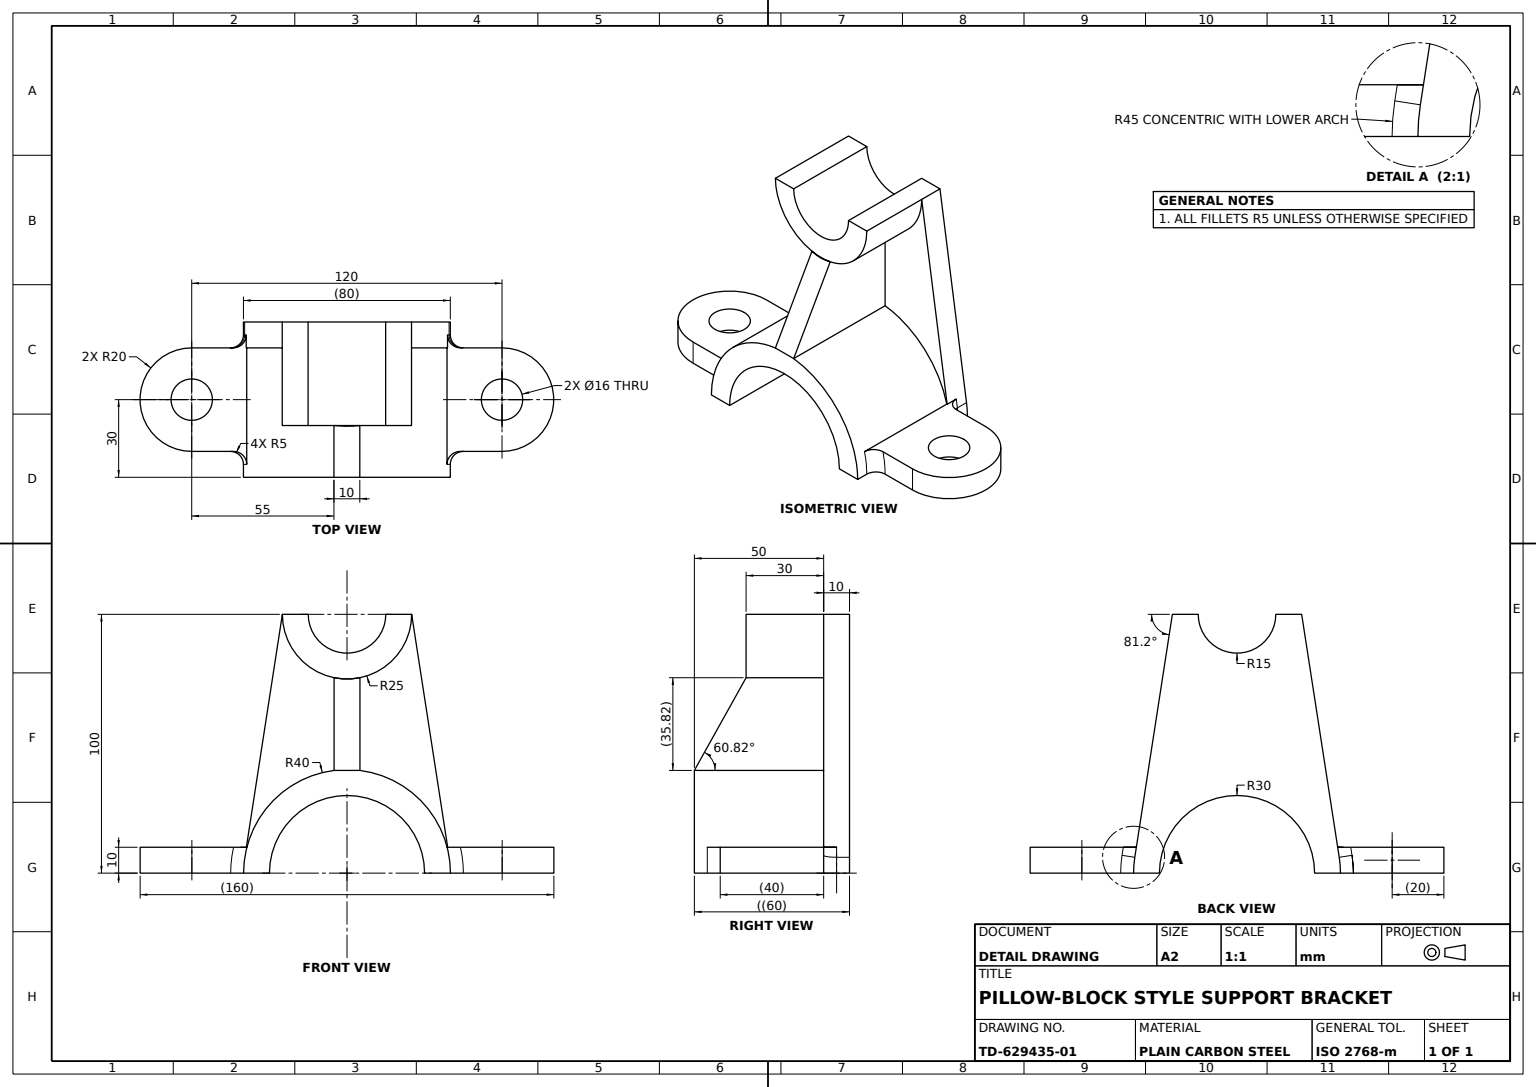
SolidWorks part; units mm, degrees
material "Plain Carbon Steel"
ref_plane "Front Plane" through (0, 0, 0) normal (0, 0, 1) x (1, 0, 0)
ref_plane "Top Plane" through (0, 0, 0) normal (0, 1, 0) x (1, 0, 0)
ref_plane "Right Plane" through (0, 0, 0) normal (1, 0, 0) x (0, 0, -1)
sketch "Base Profile Sketch" plane through (0, 0, 0) normal (0, 0, 1) x (1, 0, 0)
  line L0 (-120.4073, 0) -> (121.757, 0) construction
  line L1 (-40, 0) -> (-30, 0)
  line L2 (0, 67.9641) -> (0, -77.6044) construction
  line L3 (30, 0) -> (40, 0)
  arc A0 (40, 0) -> (-40, 0) centre (0, 0) ccw
  arc A1 (30, 0) -> (-30, 0) centre (0, 0) ccw
  dimension "D1" = 80
  dimension "D2" = 60
extrude "Base Block" add sketch "Base Profile Sketch" along normal blind 50
sketch "Upright Profile Sketch" plane through (0, 0, 50) normal (0, 0, 1) x (1, 0, 0)
  line L0 (0, 85.1126) -> (0, 0) construction
  line L1 (-65.6994, 0) -> (83.264, 0) construction
  line L2 (-55.0918, 100) -> (-15, 100) construction
  line L3 (-25, 100) -> (-15, 100)
  line L4 (15, 100) -> (25, 100)
  line L5 (15, 100) -> (96.0215, 100) construction
  arc A0 (-25, 100) -> (25, 100) centre (0, 100) ccw
  arc A1 (-15, 100) -> (15, 100) centre (0, 100) ccw
  dimension "D1" = 50
  dimension "D2" = 30
  dimension "D3" = 100
extrude "Upright Body" add sketch "Upright Profile Sketch" against normal blind 30 separate body
sketch "Saddle Flange Sketch" plane through (0, 0, 50) normal (0, 0, 1) x (1, 0, 0)
  line L0 (-25, 100) -> (-39.5294, 6.1176)
  line L1 (25, 100) -> (39.5294, 6.1176)
  arc A0 (-25, 100) -> (25, 100) centre (0, 100) ccw construction
  arc A1 (-25, 100) -> (25, 100) centre (0, 100) ccw
  arc A2 (40, 0) -> (-40, 0) centre (0, 0) ccw construction
  arc A3 (39.5294, 6.1176) -> (-39.5294, 6.1176) centre (0, 0) ccw
extrude "Saddle Flange" add sketch "Saddle Flange Sketch" along normal blind 10 separate body
sketch "Side Boss 1 Sketch" plane through (0, 0, 50) normal (0, 0, 1) x (1, 0, 0)
  line L2 (-15, 100) -> (-25, 100)
  line L3 (25, 100) -> (15, 100)
  line L4 (-15, 100) -> (-25, 100)
  line L5 (25, 100) -> (15, 100)
  arc A2 (-15, 100) -> (15, 100) centre (0, 100) ccw
  arc A3 (-25, 100) -> (25, 100) centre (0, 100) ccw
  arc A4 (-15, 100) -> (15, 100) centre (0, 100) ccw
  arc A5 (-25, 100) -> (25, 100) centre (0, 100) ccw
  dimension "D1" = 0
extrude "Side Boss 1" add sketch "Side Boss 1 Sketch" along normal blind 10
sketch "Side Boss 2 Sketch" plane through (0, 0, 50) normal (0, 0, 1) x (1, 0, 0)
  line L2 (30, 0) -> (40, 0)
  line L3 (-40, 0) -> (-30, 0)
  line L4 (30, 0) -> (40, 0)
  line L5 (-40, 0) -> (-30, 0)
  arc A2 (30, 0) -> (-30, 0) centre (0, 0) ccw
  arc A3 (40, 0) -> (-40, 0) centre (0, 0) ccw
  arc A4 (30, 0) -> (-30, 0) centre (0, 0) ccw
  arc A5 (40, 0) -> (-40, 0) centre (0, 0) ccw
  dimension "D1" = 0
extrude "Side Boss 2" add sketch "Side Boss 2 Sketch" along normal blind 10
sketch "Mounting Lug 1 Sketch" plane through (0, 0, 0) normal (0, -1, 0) x (1, 0, 0)
  line L0 (-60, 30) -> (85.4408, 30) construction
  line L1 (-40, 60) -> (-40, 0) construction
  line L2 (-40, 0) -> (-30, 0) construction
  line L3 (-60, 50) -> (-40, 50)
  line L4 (-60, 10) -> (-40, 10)
  line L5 (-40, 50) -> (-40, 10)
  arc A0 (-60, 50) -> (-60, 10) centre (-60, 30) ccw
  circle A1 centre (-60, 30) radius 8
  dimension "D1" = 40
  dimension "D2" = 16
  dimension "D3" = 30
extrude "Mounting Lug 1" add sketch "Mounting Lug 1 Sketch" against normal blind 10 separate body
sketch "Lug 1 Boss Sketch" plane through (-40, 0, 0) normal (1, 0, 0) x (0, 0, -1)
  line L4 (-50, 0) -> (-10, 0)
  line L5 (-10, 0) -> (-10, 10)
  line L6 (-10, 10) -> (-50, 10)
  line L7 (-50, 10) -> (-50, 0)
  line L8 (-50, 0) -> (-10, 0)
  line L9 (-10, 0) -> (-10, 10)
  line L10 (-10, 10) -> (-50, 10)
  line L11 (-50, 10) -> (-50, 0)
  dimension "D1" = 0
extrude "Lug 1 Boss" add sketch "Lug 1 Boss Sketch" along normal blind 5
fillet "Lug 1 Fillet R5" radius 5 3 edges at (-39.229, 8.0588, 50) (-39.8822, 3.0679, 50) (-39.6812, 5.0402, 10)
sketch "Mounting Lug 2 Sketch" plane through (0, 0, 0) normal (0, -1, 0) x (1, 0, 0)
  line L0 (-60, 30) -> (102.5211, 30) construction
  line L1 (40, 60) -> (40, 0) construction
  line L2 (60, 50) -> (40, 50)
  line L3 (60, 10) -> (40, 10)
  line L4 (40, 50) -> (40, 10)
  circle A0 centre (60, 30) radius 8
  arc A1 (60, 10) -> (60, 50) centre (60, 30) ccw
  dimension "D1" = 40
  dimension "D2" = 16
extrude "Mounting Lug 2" add sketch "Mounting Lug 2 Sketch" against normal blind 10 separate body
sketch "Lug 2 Boss Sketch" plane through (40, 0, 0) normal (-1, 0, 0) x (0, 0, 1)
  line L4 (10, 0) -> (50, 0)
  line L5 (50, 0) -> (50, 10)
  line L6 (50, 10) -> (10, 10)
  line L7 (10, 10) -> (10, 0)
  line L8 (10, 0) -> (50, 0)
  line L9 (50, 0) -> (50, 10)
  line L10 (50, 10) -> (10, 10)
  line L11 (10, 10) -> (10, 0)
  dimension "D1" = 0
extrude "Lug 2 Boss" add sketch "Lug 2 Boss Sketch" along normal blind 5
fillet "Lug 2 Fillet R5" radius 5 3 edges at (39.6812, 5.0402, 10) (39.8822, 3.0679, 50) (39.229, 8.0588, 50)
sketch "Side Rib Sketch" plane through (0, 0, 50) normal (0, 0, -1) x (-1, 0, 0)
  line L0 (0, 242.8634) -> (0, -20.4744) construction
  line L3 (-5, 75.5051) -> (-5, 39.6863)
  line L5 (5, 75.5051) -> (5, 39.6863)
  arc A0 (-25, 100) -> (25, 100) centre (0, 100) ccw construction
  arc A1 (-5, 75.5051) -> (5, 75.5051) centre (0, 100) ccw
  arc A2 (38.7298, 10) -> (-38.7298, 10) centre (0, 0) ccw construction
  arc A3 (5, 39.6863) -> (-5, 39.6863) centre (0, 0) ccw
  point P4 (0, 111.1945)
  point P7 (0, 57.3431)
  dimension "D1" = 10
  dimension "D2" = 35.8188
  dimension "D3" = 20.4744
  dimension "D4" = 263.3378
  dimension "D5" = 57.3431
extrude "Side Rib" add sketch "Side Rib Sketch" along normal up to surface (50 mm away)
sketch "Rib Relief Cut Sketch" plane through (-5, 0, 0) normal (-1, 0, 0) x (0, 0, 1)
  line L0 (20, 75.5051) -> (0, 39.6863)
  line L5 (20, 75.5051) -> (0, 75.5051)
  line L6 (0, 75.5051) -> (0, 39.6863)
  line L7 (0, 39.6863) -> (50, 39.6863)
  line L8 (50, 39.6863) -> (50, 75.5051)
  line L9 (50, 75.5051) -> (20, 75.5051)
  line L10 (20, 75.5051) -> (0, 75.5051)
  line L11 (0, 75.5051) -> (0, 39.6863)
  dimension "D1" = 0
extrude "Rib Relief Cut" cut sketch "Rib Relief Cut Sketch" against normal blind 15
